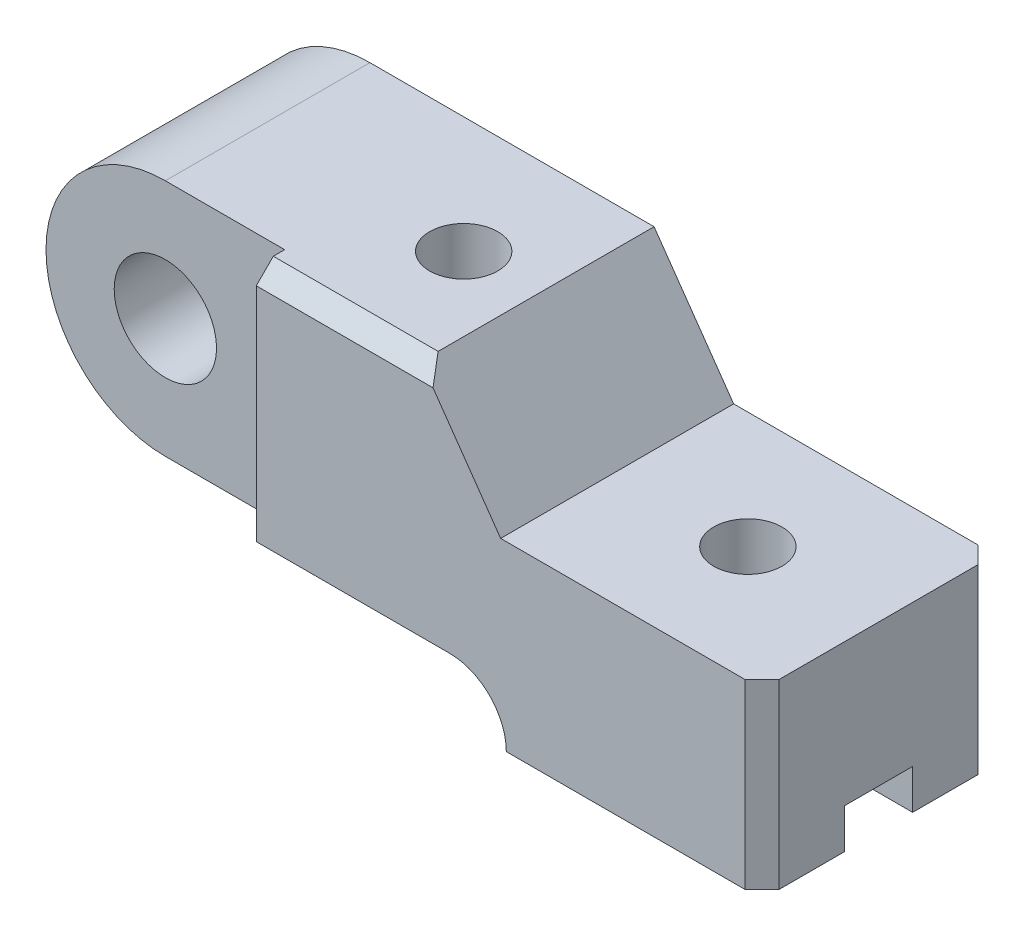
ISO-10303-21;
HEADER;
FILE_DESCRIPTION(('STEP AP214'),'2;1');
FILE_NAME('part.step','',(''),(''),'','','');
FILE_SCHEMA(('AUTOMOTIVE_DESIGN { 1 0 10303 214 1 1 1 1 }'));
ENDSEC;
DATA;
#1=APPLICATION_CONTEXT('core data for automotive mechanical design processes');
#2=APPLICATION_PROTOCOL_DEFINITION('international standard','automotive_design',2000,#1);
#3=PRODUCT_CONTEXT('',#1,'mechanical');
#4=PRODUCT('Part','Part','',(#3));
#5=PRODUCT_RELATED_PRODUCT_CATEGORY('part','',(#4));
#6=PRODUCT_DEFINITION_FORMATION('','',#4);
#7=PRODUCT_DEFINITION_CONTEXT('part definition',#1,'design');
#8=PRODUCT_DEFINITION('design','',#6,#7);
#9=PRODUCT_DEFINITION_SHAPE('','',#8);
#10=(LENGTH_UNIT() NAMED_UNIT(*) SI_UNIT(.MILLI.,.METRE.));
#11=(NAMED_UNIT(*) PLANE_ANGLE_UNIT() SI_UNIT($,.RADIAN.));
#12=(NAMED_UNIT(*) SI_UNIT($,.STERADIAN.) SOLID_ANGLE_UNIT());
#13=UNCERTAINTY_MEASURE_WITH_UNIT(LENGTH_MEASURE(1.E-05),#10,'distance_accuracy_value','');
#14=(GEOMETRIC_REPRESENTATION_CONTEXT(3) GLOBAL_UNCERTAINTY_ASSIGNED_CONTEXT((#13)) GLOBAL_UNIT_ASSIGNED_CONTEXT((#10,
#11,#12)) REPRESENTATION_CONTEXT('',''));
#15=CARTESIAN_POINT('',(0.,0.,0.));
#16=DIRECTION('',(0.,0.,1.));
#17=DIRECTION('',(1.,0.,0.));
#18=AXIS2_PLACEMENT_3D('',#15,#16,#17);
#19=CARTESIAN_POINT('',(0.,0.,20.5));
#20=DIRECTION('',(0.,1.,0.));
#21=DIRECTION('',(-1.,0.,0.));
#22=AXIS2_PLACEMENT_3D('',#19,#20,#21);
#23=PLANE('',#22);
#24=DIRECTION('',(0.,0.,-1.));
#25=VECTOR('',#24,1.);
#26=CARTESIAN_POINT('',(0.,0.,20.5));
#27=LINE('',#26,#25);
#28=CARTESIAN_POINT('',(0.,0.,17.5));
#29=VERTEX_POINT('',#28);
#30=CARTESIAN_POINT('',(0.,0.,6.));
#31=VERTEX_POINT('',#30);
#32=EDGE_CURVE('E195',#29,#31,#27,.T.);
#33=ORIENTED_EDGE('',*,*,#32,.F.);
#34=DIRECTION('',(-0.707106781186546,0.,0.707106781186549));
#35=VECTOR('',#34,1.);
#36=CARTESIAN_POINT('',(-3.,0.,20.5));
#37=LINE('',#36,#35);
#38=CARTESIAN_POINT('',(-3.,0.,20.5));
#39=VERTEX_POINT('',#38);
#40=EDGE_CURVE('E260',#29,#39,#37,.T.);
#41=ORIENTED_EDGE('',*,*,#40,.T.);
#42=DIRECTION('',(1.,0.,0.));
#43=VECTOR('',#42,1.);
#44=CARTESIAN_POINT('',(0.,0.,20.5));
#45=LINE('',#44,#43);
#46=CARTESIAN_POINT('',(-45.,0.,20.5));
#47=VERTEX_POINT('',#46);
#48=EDGE_CURVE('E191',#47,#39,#45,.T.);
#49=ORIENTED_EDGE('',*,*,#48,.F.);
#50=DIRECTION('',(0.,0.,-1.));
#51=VECTOR('',#50,1.);
#52=CARTESIAN_POINT('',(-45.,0.,20.5));
#53=LINE('',#52,#51);
#54=CARTESIAN_POINT('',(-45.,0.,6.));
#55=VERTEX_POINT('',#54);
#56=EDGE_CURVE('E202',#47,#55,#53,.T.);
#57=ORIENTED_EDGE('',*,*,#56,.T.);
#58=DIRECTION('',(1.,0.,0.));
#59=VECTOR('',#58,1.);
#60=CARTESIAN_POINT('',(-131.,0.,6.));
#61=LINE('',#60,#59);
#62=EDGE_CURVE('E326',#55,#31,#61,.T.);
#63=ORIENTED_EDGE('',*,*,#62,.T.);
#64=EDGE_LOOP('',(#33,#41,#49,#57,#63));
#65=FACE_BOUND('',#64,.T.);
#66=ADVANCED_FACE('F41',(#65),#23,.F.);
#67=CARTESIAN_POINT('',(-55.,0.,20.5));
#68=DIRECTION('',(0.,0.,1.));
#69=DIRECTION('',(1.,0.,0.));
#70=AXIS2_PLACEMENT_3D('',#67,#68,#69);
#71=PLANE('',#70);
#72=ORIENTED_EDGE('',*,*,#48,.T.);
#73=DIRECTION('',(0.,1.,0.));
#74=VECTOR('',#73,1.);
#75=CARTESIAN_POINT('',(-3.,32.,20.5));
#76=LINE('',#75,#74);
#77=CARTESIAN_POINT('',(-3.,32.,20.5));
#78=VERTEX_POINT('',#77);
#79=EDGE_CURVE('E255',#39,#78,#76,.T.);
#80=ORIENTED_EDGE('',*,*,#79,.T.);
#81=DIRECTION('',(-1.,0.,0.));
#82=VECTOR('',#81,1.);
#83=CARTESIAN_POINT('',(-45.9968419909216,32.,20.5));
#84=LINE('',#83,#82);
#85=CARTESIAN_POINT('',(-45.9968419909216,32.,20.5));
#86=VERTEX_POINT('',#85);
#87=EDGE_CURVE('E280',#78,#86,#84,.T.);
#88=ORIENTED_EDGE('',*,*,#87,.T.);
#89=DIRECTION('',(-0.573576436351044,0.819152044288993,0.));
#90=VECTOR('',#89,1.);
#91=CARTESIAN_POINT('',(-60.,51.9985821987602,20.5));
#92=LINE('',#91,#90);
#93=CARTESIAN_POINT('',(-57.8993773853709,48.9985821987602,20.5));
#94=VERTEX_POINT('',#93);
#95=EDGE_CURVE('E306',#86,#94,#92,.T.);
#96=ORIENTED_EDGE('',*,*,#95,.T.);
#97=DIRECTION('',(-1.,0.,0.));
#98=VECTOR('',#97,1.);
#99=CARTESIAN_POINT('',(-89.,48.9985821987602,20.5));
#100=LINE('',#99,#98);
#101=CARTESIAN_POINT('',(-89.,48.9985821987602,20.5));
#102=VERTEX_POINT('',#101);
#103=EDGE_CURVE('E253',#94,#102,#100,.T.);
#104=ORIENTED_EDGE('',*,*,#103,.T.);
#105=DIRECTION('',(0.,1.,0.));
#106=VECTOR('',#105,1.);
#107=CARTESIAN_POINT('',(-89.,0.,20.5));
#108=LINE('',#107,#106);
#109=CARTESIAN_POINT('',(-89.,9.99858219876021,20.5));
#110=VERTEX_POINT('',#109);
#111=EDGE_CURVE('E318',#110,#102,#108,.T.);
#112=ORIENTED_EDGE('',*,*,#111,.F.);
#113=DIRECTION('',(1.,0.,0.));
#114=VECTOR('',#113,1.);
#115=CARTESIAN_POINT('',(-110.,9.99858219876022,20.5));
#116=LINE('',#115,#114);
#117=CARTESIAN_POINT('',(-55.1683865037197,9.99858219876023,20.5));
#118=VERTEX_POINT('',#117);
#119=EDGE_CURVE('E313',#110,#118,#116,.T.);
#120=ORIENTED_EDGE('',*,*,#119,.T.);
#121=CARTESIAN_POINT('',(-55.,0.,20.5));
#122=DIRECTION('',(0.,0.,-1.));
#123=DIRECTION('',(1.,0.,0.));
#124=AXIS2_PLACEMENT_3D('',#121,#122,#123);
#125=CIRCLE('',#124,10.);
#126=EDGE_CURVE('E200',#118,#47,#125,.T.);
#127=ORIENTED_EDGE('',*,*,#126,.T.);
#128=EDGE_LOOP('',(#72,#80,#88,#96,#104,#112,#120,#127));
#129=FACE_BOUND('',#128,.T.);
#130=ADVANCED_FACE('F268',(#129),#71,.T.);
#131=CARTESIAN_POINT('',(-55.,0.,-20.5));
#132=DIRECTION('',(0.,0.,1.));
#133=DIRECTION('',(1.,0.,0.));
#134=AXIS2_PLACEMENT_3D('',#131,#132,#133);
#135=PLANE('',#134);
#136=DIRECTION('',(-1.,0.,0.));
#137=VECTOR('',#136,1.);
#138=CARTESIAN_POINT('',(-45.9968419909216,32.,-20.5));
#139=LINE('',#138,#137);
#140=CARTESIAN_POINT('',(-3.00000000000002,32.,-20.5));
#141=VERTEX_POINT('',#140);
#142=CARTESIAN_POINT('',(-45.9968419909216,32.,-20.5));
#143=VERTEX_POINT('',#142);
#144=EDGE_CURVE('E285',#141,#143,#139,.T.);
#145=ORIENTED_EDGE('',*,*,#144,.F.);
#146=DIRECTION('',(0.,-1.,0.));
#147=VECTOR('',#146,1.);
#148=CARTESIAN_POINT('',(-3.00000000000002,0.,-20.5));
#149=LINE('',#148,#147);
#150=CARTESIAN_POINT('',(-3.00000000000002,0.,-20.5));
#151=VERTEX_POINT('',#150);
#152=EDGE_CURVE('E247',#141,#151,#149,.T.);
#153=ORIENTED_EDGE('',*,*,#152,.T.);
#154=DIRECTION('',(1.,0.,0.));
#155=VECTOR('',#154,1.);
#156=CARTESIAN_POINT('',(0.,0.,-20.5));
#157=LINE('',#156,#155);
#158=CARTESIAN_POINT('',(-45.,0.,-20.5));
#159=VERTEX_POINT('',#158);
#160=EDGE_CURVE('E201',#159,#151,#157,.T.);
#161=ORIENTED_EDGE('',*,*,#160,.F.);
#162=CARTESIAN_POINT('',(-55.,0.,-20.5));
#163=DIRECTION('',(0.,0.,-1.));
#164=DIRECTION('',(1.,0.,0.));
#165=AXIS2_PLACEMENT_3D('',#162,#163,#164);
#166=CIRCLE('',#165,10.);
#167=CARTESIAN_POINT('',(-55.1683865037197,9.99858219876023,-20.5));
#168=VERTEX_POINT('',#167);
#169=EDGE_CURVE('E305',#168,#159,#166,.T.);
#170=ORIENTED_EDGE('',*,*,#169,.F.);
#171=DIRECTION('',(1.,0.,0.));
#172=VECTOR('',#171,1.);
#173=CARTESIAN_POINT('',(-55.1683865037197,9.99858219876023,-20.5));
#174=LINE('',#173,#172);
#175=CARTESIAN_POINT('',(-110.,9.99858219876022,-20.5));
#176=VERTEX_POINT('',#175);
#177=EDGE_CURVE('E302',#176,#168,#174,.T.);
#178=ORIENTED_EDGE('',*,*,#177,.F.);
#179=CARTESIAN_POINT('',(-110.,30.9985821987602,-20.5));
#180=DIRECTION('',(0.,0.,1.));
#181=DIRECTION('',(1.,0.,0.));
#182=AXIS2_PLACEMENT_3D('',#179,#180,#181);
#183=CIRCLE('',#182,21.);
#184=CARTESIAN_POINT('',(-110.,51.9985821987602,-20.5));
#185=VERTEX_POINT('',#184);
#186=EDGE_CURVE('E299',#185,#176,#183,.T.);
#187=ORIENTED_EDGE('',*,*,#186,.F.);
#188=DIRECTION('',(-1.,0.,0.));
#189=VECTOR('',#188,1.);
#190=CARTESIAN_POINT('',(-110.,51.9985821987602,-20.5));
#191=LINE('',#190,#189);
#192=CARTESIAN_POINT('',(-60.,51.9985821987602,-20.5));
#193=VERTEX_POINT('',#192);
#194=EDGE_CURVE('E295',#193,#185,#191,.T.);
#195=ORIENTED_EDGE('',*,*,#194,.F.);
#196=DIRECTION('',(-0.573576436351044,0.819152044288993,0.));
#197=VECTOR('',#196,1.);
#198=CARTESIAN_POINT('',(-60.,51.9985821987602,-20.5));
#199=LINE('',#198,#197);
#200=EDGE_CURVE('E286',#143,#193,#199,.T.);
#201=ORIENTED_EDGE('',*,*,#200,.F.);
#202=EDGE_LOOP('',(#145,#153,#161,#170,#178,#187,#195,#201));
#203=FACE_BOUND('',#202,.T.);
#204=CARTESIAN_POINT('',(-110.,30.9985821987602,-20.5));
#205=DIRECTION('',(0.,0.,1.));
#206=DIRECTION('',(1.,0.,0.));
#207=AXIS2_PLACEMENT_3D('',#204,#205,#206);
#208=CIRCLE('',#207,9.);
#209=CARTESIAN_POINT('',(-101.,30.9985821987602,-20.5));
#210=VERTEX_POINT('',#209);
#211=EDGE_CURVE('E234',#210,#210,#208,.T.);
#212=ORIENTED_EDGE('',*,*,#211,.T.);
#213=EDGE_LOOP('',(#212));
#214=FACE_BOUND('',#213,.T.);
#215=ADVANCED_FACE('F284',(#203,#214),#135,.F.);
#216=CARTESIAN_POINT('',(0.,32.,20.5));
#217=DIRECTION('',(-1.,0.,0.));
#218=DIRECTION('',(0.,0.,1.));
#219=AXIS2_PLACEMENT_3D('',#216,#217,#218);
#220=PLANE('',#219);
#221=CARTESIAN_POINT('',(0.,0.,-6.));
#222=VERTEX_POINT('',#221);
#223=CARTESIAN_POINT('',(0.,0.,-17.5));
#224=VERTEX_POINT('',#223);
#225=EDGE_CURVE('E184',#222,#224,#27,.T.);
#226=ORIENTED_EDGE('',*,*,#225,.T.);
#227=DIRECTION('',(0.,1.,0.));
#228=VECTOR('',#227,1.);
#229=CARTESIAN_POINT('',(0.,32.,-17.5));
#230=LINE('',#229,#228);
#231=CARTESIAN_POINT('',(0.,32.,-17.5));
#232=VERTEX_POINT('',#231);
#233=EDGE_CURVE('E245',#224,#232,#230,.T.);
#234=ORIENTED_EDGE('',*,*,#233,.T.);
#235=DIRECTION('',(0.,0.,-1.));
#236=VECTOR('',#235,1.);
#237=CARTESIAN_POINT('',(0.,32.,20.5));
#238=LINE('',#237,#236);
#239=CARTESIAN_POINT('',(0.,32.,17.5));
#240=VERTEX_POINT('',#239);
#241=EDGE_CURVE('E219',#240,#232,#238,.T.);
#242=ORIENTED_EDGE('',*,*,#241,.F.);
#243=DIRECTION('',(0.,-1.,0.));
#244=VECTOR('',#243,1.);
#245=CARTESIAN_POINT('',(0.,0.,17.5));
#246=LINE('',#245,#244);
#247=EDGE_CURVE('E238',#240,#29,#246,.T.);
#248=ORIENTED_EDGE('',*,*,#247,.T.);
#249=ORIENTED_EDGE('',*,*,#32,.T.);
#250=DIRECTION('',(0.,-1.,0.));
#251=VECTOR('',#250,1.);
#252=CARTESIAN_POINT('',(0.,0.,6.));
#253=LINE('',#252,#251);
#254=CARTESIAN_POINT('',(0.,7.,6.));
#255=VERTEX_POINT('',#254);
#256=EDGE_CURVE('E177',#255,#31,#253,.T.);
#257=ORIENTED_EDGE('',*,*,#256,.F.);
#258=DIRECTION('',(0.,0.,1.));
#259=VECTOR('',#258,1.);
#260=CARTESIAN_POINT('',(0.,7.,6.));
#261=LINE('',#260,#259);
#262=CARTESIAN_POINT('',(0.,7.,-6.));
#263=VERTEX_POINT('',#262);
#264=EDGE_CURVE('E186',#263,#255,#261,.T.);
#265=ORIENTED_EDGE('',*,*,#264,.F.);
#266=DIRECTION('',(0.,1.,0.));
#267=VECTOR('',#266,1.);
#268=CARTESIAN_POINT('',(0.,7.,-6.));
#269=LINE('',#268,#267);
#270=EDGE_CURVE('E166',#222,#263,#269,.T.);
#271=ORIENTED_EDGE('',*,*,#270,.F.);
#272=EDGE_LOOP('',(#226,#234,#242,#248,#249,#257,#265,#271));
#273=FACE_BOUND('',#272,.T.);
#274=ADVANCED_FACE('F185',(#273),#220,.F.);
#275=CARTESIAN_POINT('',(-45.9968419909216,32.,20.5));
#276=DIRECTION('',(0.,-1.,0.));
#277=DIRECTION('',(1.,0.,0.));
#278=AXIS2_PLACEMENT_3D('',#275,#276,#277);
#279=PLANE('',#278);
#280=CARTESIAN_POINT('',(-22.9984209954608,32.,0.));
#281=DIRECTION('',(0.,-1.,0.));
#282=DIRECTION('',(1.,0.,0.));
#283=AXIS2_PLACEMENT_3D('',#280,#281,#282);
#284=CIRCLE('',#283,6.);
#285=CARTESIAN_POINT('',(-16.9984209954608,32.,0.));
#286=VERTEX_POINT('',#285);
#287=EDGE_CURVE('E232',#286,#286,#284,.T.);
#288=ORIENTED_EDGE('',*,*,#287,.T.);
#289=EDGE_LOOP('',(#288));
#290=FACE_BOUND('',#289,.T.);
#291=ORIENTED_EDGE('',*,*,#241,.T.);
#292=DIRECTION('',(0.707106781186549,0.,0.707106781186546));
#293=VECTOR('',#292,1.);
#294=CARTESIAN_POINT('',(0.,32.,-17.5));
#295=LINE('',#294,#293);
#296=EDGE_CURVE('E248',#232,#141,#295,.F.);
#297=ORIENTED_EDGE('',*,*,#296,.T.);
#298=ORIENTED_EDGE('',*,*,#144,.T.);
#299=DIRECTION('',(0.,0.,-1.));
#300=VECTOR('',#299,1.);
#301=CARTESIAN_POINT('',(-45.9968419909216,32.,20.5));
#302=LINE('',#301,#300);
#303=EDGE_CURVE('E220',#86,#143,#302,.T.);
#304=ORIENTED_EDGE('',*,*,#303,.F.);
#305=ORIENTED_EDGE('',*,*,#87,.F.);
#306=DIRECTION('',(0.707106781186546,0.,-0.707106781186549));
#307=VECTOR('',#306,1.);
#308=CARTESIAN_POINT('',(-3.,32.,20.5));
#309=LINE('',#308,#307);
#310=EDGE_CURVE('E242',#78,#240,#309,.T.);
#311=ORIENTED_EDGE('',*,*,#310,.T.);
#312=EDGE_LOOP('',(#291,#297,#298,#304,#305,#311));
#313=FACE_BOUND('',#312,.T.);
#314=ADVANCED_FACE('F274',(#290,#313),#279,.F.);
#315=CARTESIAN_POINT('',(-60.,51.9985821987602,20.5));
#316=DIRECTION('',(-0.819152044288993,-0.573576436351044,0.));
#317=DIRECTION('',(0.573576436351044,-0.819152044288993,0.));
#318=AXIS2_PLACEMENT_3D('',#315,#316,#317);
#319=PLANE('',#318);
#320=DIRECTION('',(0.,0.,-1.));
#321=VECTOR('',#320,1.);
#322=CARTESIAN_POINT('',(-60.,51.9985821987602,20.5));
#323=LINE('',#322,#321);
#324=CARTESIAN_POINT('',(-60.,51.9985821987602,17.5));
#325=VERTEX_POINT('',#324);
#326=EDGE_CURVE('E214',#325,#193,#323,.T.);
#327=ORIENTED_EDGE('',*,*,#326,.F.);
#328=DIRECTION('',(0.443712606279655,-0.633687274224641,0.633687274224644));
#329=VECTOR('',#328,1.);
#330=CARTESIAN_POINT('',(-57.3285454230678,48.1833496696123,21.3152325291479));
#331=LINE('',#330,#329);
#332=EDGE_CURVE('E11',#325,#94,#331,.T.);
#333=ORIENTED_EDGE('',*,*,#332,.T.);
#334=ORIENTED_EDGE('',*,*,#95,.F.);
#335=ORIENTED_EDGE('',*,*,#303,.T.);
#336=ORIENTED_EDGE('',*,*,#200,.T.);
#337=EDGE_LOOP('',(#327,#333,#334,#335,#336));
#338=FACE_BOUND('',#337,.T.);
#339=ADVANCED_FACE('F409',(#338),#319,.F.);
#340=CARTESIAN_POINT('',(-110.,51.9985821987602,20.5));
#341=DIRECTION('',(0.,-1.,0.));
#342=DIRECTION('',(0.,0.,-1.));
#343=AXIS2_PLACEMENT_3D('',#340,#341,#342);
#344=PLANE('',#343);
#345=CARTESIAN_POINT('',(-72.9984209954608,51.9985821987602,0.));
#346=DIRECTION('',(0.,1.,0.));
#347=DIRECTION('',(0.,0.,1.));
#348=AXIS2_PLACEMENT_3D('',#345,#346,#347);
#349=CIRCLE('',#348,6.);
#350=CARTESIAN_POINT('',(-72.9984209954608,51.9985821987602,6.));
#351=VERTEX_POINT('',#350);
#352=EDGE_CURVE('E226',#351,#351,#349,.T.);
#353=ORIENTED_EDGE('',*,*,#352,.F.);
#354=EDGE_LOOP('',(#353));
#355=FACE_BOUND('',#354,.T.);
#356=DIRECTION('',(0.,0.,-1.));
#357=VECTOR('',#356,1.);
#358=CARTESIAN_POINT('',(-89.,51.9985821987602,15.5));
#359=LINE('',#358,#357);
#360=CARTESIAN_POINT('',(-89.,51.9985821987602,17.5));
#361=VERTEX_POINT('',#360);
#362=CARTESIAN_POINT('',(-89.,51.9985821987602,15.5));
#363=VERTEX_POINT('',#362);
#364=EDGE_CURVE('E345',#361,#363,#359,.T.);
#365=ORIENTED_EDGE('',*,*,#364,.F.);
#366=DIRECTION('',(1.,0.,0.));
#367=VECTOR('',#366,1.);
#368=CARTESIAN_POINT('',(-60.,51.9985821987602,17.5));
#369=LINE('',#368,#367);
#370=EDGE_CURVE('E49',#361,#325,#369,.T.);
#371=ORIENTED_EDGE('',*,*,#370,.T.);
#372=ORIENTED_EDGE('',*,*,#326,.T.);
#373=ORIENTED_EDGE('',*,*,#194,.T.);
#374=DIRECTION('',(0.,0.,-1.));
#375=VECTOR('',#374,1.);
#376=CARTESIAN_POINT('',(-110.,51.9985821987602,20.5));
#377=LINE('',#376,#375);
#378=CARTESIAN_POINT('',(-110.,51.9985821987602,15.5));
#379=VERTEX_POINT('',#378);
#380=EDGE_CURVE('E213',#379,#185,#377,.T.);
#381=ORIENTED_EDGE('',*,*,#380,.F.);
#382=DIRECTION('',(-1.,0.,0.));
#383=VECTOR('',#382,1.);
#384=CARTESIAN_POINT('',(-131.,51.9985821987602,15.5));
#385=LINE('',#384,#383);
#386=EDGE_CURVE('E347',#363,#379,#385,.T.);
#387=ORIENTED_EDGE('',*,*,#386,.F.);
#388=EDGE_LOOP('',(#365,#371,#372,#373,#381,#387));
#389=FACE_BOUND('',#388,.T.);
#390=ADVANCED_FACE('F410',(#355,#389),#344,.F.);
#391=CARTESIAN_POINT('',(-110.,30.9985821987602,20.5));
#392=DIRECTION('',(0.,0.,-1.));
#393=DIRECTION('',(-1.,0.,0.));
#394=AXIS2_PLACEMENT_3D('',#391,#392,#393);
#395=CYLINDRICAL_SURFACE('',#394,21.);
#396=CARTESIAN_POINT('',(-110.,30.9985821987602,15.5));
#397=DIRECTION('',(0.,0.,-1.));
#398=DIRECTION('',(-1.,0.,0.));
#399=AXIS2_PLACEMENT_3D('',#396,#397,#398);
#400=CIRCLE('',#399,21.);
#401=CARTESIAN_POINT('',(-110.,9.99858219876021,15.5));
#402=VERTEX_POINT('',#401);
#403=EDGE_CURVE('E359',#402,#379,#400,.T.);
#404=ORIENTED_EDGE('',*,*,#403,.T.);
#405=ORIENTED_EDGE('',*,*,#380,.T.);
#406=ORIENTED_EDGE('',*,*,#186,.T.);
#407=DIRECTION('',(0.,0.,-1.));
#408=VECTOR('',#407,1.);
#409=CARTESIAN_POINT('',(-110.,9.99858219876022,20.5));
#410=LINE('',#409,#408);
#411=EDGE_CURVE('E211',#402,#176,#410,.T.);
#412=ORIENTED_EDGE('',*,*,#411,.F.);
#413=EDGE_LOOP('',(#404,#405,#406,#412));
#414=FACE_BOUND('',#413,.T.);
#415=ADVANCED_FACE('F402',(#414),#395,.T.);
#416=CARTESIAN_POINT('',(-55.1683865037197,9.99858219876023,20.5));
#417=DIRECTION('',(0.,1.,0.));
#418=DIRECTION('',(-1.,0.,0.));
#419=AXIS2_PLACEMENT_3D('',#416,#417,#418);
#420=PLANE('',#419);
#421=CARTESIAN_POINT('',(-72.9984209954608,9.99858219876023,0.));
#422=DIRECTION('',(0.,1.,0.));
#423=DIRECTION('',(-1.,0.,0.));
#424=AXIS2_PLACEMENT_3D('',#421,#422,#423);
#425=CIRCLE('',#424,6.);
#426=CARTESIAN_POINT('',(-78.9984209954608,9.99858219876022,0.));
#427=VERTEX_POINT('',#426);
#428=EDGE_CURVE('E227',#427,#427,#425,.T.);
#429=ORIENTED_EDGE('',*,*,#428,.T.);
#430=EDGE_LOOP('',(#429));
#431=FACE_BOUND('',#430,.T.);
#432=DIRECTION('',(0.,0.,-1.));
#433=VECTOR('',#432,1.);
#434=CARTESIAN_POINT('',(-89.,9.99858219876022,20.5));
#435=LINE('',#434,#433);
#436=CARTESIAN_POINT('',(-89.,9.99858219876022,15.5));
#437=VERTEX_POINT('',#436);
#438=EDGE_CURVE('E224',#110,#437,#435,.T.);
#439=ORIENTED_EDGE('',*,*,#438,.T.);
#440=DIRECTION('',(-1.,0.,0.));
#441=VECTOR('',#440,1.);
#442=CARTESIAN_POINT('',(-55.1683865037197,9.99858219876023,15.5));
#443=LINE('',#442,#441);
#444=EDGE_CURVE('E230',#437,#402,#443,.T.);
#445=ORIENTED_EDGE('',*,*,#444,.T.);
#446=ORIENTED_EDGE('',*,*,#411,.T.);
#447=ORIENTED_EDGE('',*,*,#177,.T.);
#448=DIRECTION('',(0.,0.,-1.));
#449=VECTOR('',#448,1.);
#450=CARTESIAN_POINT('',(-55.1683865037197,9.99858219876023,20.5));
#451=LINE('',#450,#449);
#452=EDGE_CURVE('E208',#118,#168,#451,.T.);
#453=ORIENTED_EDGE('',*,*,#452,.F.);
#454=ORIENTED_EDGE('',*,*,#119,.F.);
#455=EDGE_LOOP('',(#439,#445,#446,#447,#453,#454));
#456=FACE_BOUND('',#455,.T.);
#457=ADVANCED_FACE('F319',(#431,#456),#420,.F.);
#458=CARTESIAN_POINT('',(-55.,0.,20.5));
#459=DIRECTION('',(0.,0.,-1.));
#460=DIRECTION('',(-1.,0.,0.));
#461=AXIS2_PLACEMENT_3D('',#458,#459,#460);
#462=CYLINDRICAL_SURFACE('',#461,10.);
#463=DIRECTION('',(0.,0.,-1.));
#464=VECTOR('',#463,1.);
#465=CARTESIAN_POINT('',(-47.8585715714571,7.,20.5));
#466=LINE('',#465,#464);
#467=CARTESIAN_POINT('',(-47.8585715714571,7.,-6.));
#468=VERTEX_POINT('',#467);
#469=CARTESIAN_POINT('',(-47.8585715714571,7.,6.));
#470=VERTEX_POINT('',#469);
#471=EDGE_CURVE('E343',#468,#470,#466,.F.);
#472=ORIENTED_EDGE('',*,*,#471,.T.);
#473=CARTESIAN_POINT('',(-55.,0.,6.));
#474=DIRECTION('',(0.,0.,1.));
#475=DIRECTION('',(1.,0.,0.));
#476=AXIS2_PLACEMENT_3D('',#473,#474,#475);
#477=CIRCLE('',#476,10.);
#478=EDGE_CURVE('E324',#470,#55,#477,.F.);
#479=ORIENTED_EDGE('',*,*,#478,.T.);
#480=ORIENTED_EDGE('',*,*,#56,.F.);
#481=ORIENTED_EDGE('',*,*,#126,.F.);
#482=ORIENTED_EDGE('',*,*,#452,.T.);
#483=ORIENTED_EDGE('',*,*,#169,.T.);
#484=CARTESIAN_POINT('',(-45.,0.,-6.));
#485=VERTEX_POINT('',#484);
#486=EDGE_CURVE('E197',#485,#159,#53,.T.);
#487=ORIENTED_EDGE('',*,*,#486,.F.);
#488=CARTESIAN_POINT('',(-55.,0.,-6.));
#489=DIRECTION('',(0.,0.,-1.));
#490=DIRECTION('',(-1.,0.,0.));
#491=AXIS2_PLACEMENT_3D('',#488,#489,#490);
#492=CIRCLE('',#491,10.);
#493=EDGE_CURVE('E171',#485,#468,#492,.F.);
#494=ORIENTED_EDGE('',*,*,#493,.T.);
#495=EDGE_LOOP('',(#472,#479,#480,#481,#482,#483,#487,#494));
#496=FACE_BOUND('',#495,.T.);
#497=ADVANCED_FACE('F323',(#496),#462,.F.);
#498=ORIENTED_EDGE('',*,*,#160,.T.);
#499=DIRECTION('',(-0.707106781186549,0.,-0.707106781186546));
#500=VECTOR('',#499,1.);
#501=CARTESIAN_POINT('',(0.,0.,-17.5));
#502=LINE('',#501,#500);
#503=EDGE_CURVE('E192',#151,#224,#502,.F.);
#504=ORIENTED_EDGE('',*,*,#503,.T.);
#505=ORIENTED_EDGE('',*,*,#225,.F.);
#506=DIRECTION('',(1.,0.,0.));
#507=VECTOR('',#506,1.);
#508=CARTESIAN_POINT('',(-131.,0.,-6.));
#509=LINE('',#508,#507);
#510=EDGE_CURVE('E164',#485,#222,#509,.T.);
#511=ORIENTED_EDGE('',*,*,#510,.F.);
#512=ORIENTED_EDGE('',*,*,#486,.T.);
#513=EDGE_LOOP('',(#498,#504,#505,#511,#512));
#514=FACE_BOUND('',#513,.T.);
#515=ADVANCED_FACE('F193',(#514),#23,.F.);
#516=CARTESIAN_POINT('',(-110.,30.9985821987602,20.5));
#517=DIRECTION('',(0.,0.,-1.));
#518=DIRECTION('',(-1.,0.,0.));
#519=AXIS2_PLACEMENT_3D('',#516,#517,#518);
#520=CYLINDRICAL_SURFACE('',#519,9.);
#521=CARTESIAN_POINT('',(-110.,30.9985821987602,15.5));
#522=DIRECTION('',(0.,0.,-1.));
#523=DIRECTION('',(-1.,0.,0.));
#524=AXIS2_PLACEMENT_3D('',#521,#522,#523);
#525=CIRCLE('',#524,9.);
#526=CARTESIAN_POINT('',(-119.,30.9985821987602,15.5));
#527=VERTEX_POINT('',#526);
#528=EDGE_CURVE('E221',#527,#527,#525,.T.);
#529=ORIENTED_EDGE('',*,*,#528,.F.);
#530=EDGE_LOOP('',(#529));
#531=FACE_BOUND('',#530,.T.);
#532=ORIENTED_EDGE('',*,*,#211,.F.);
#533=EDGE_LOOP('',(#532));
#534=FACE_BOUND('',#533,.T.);
#535=ADVANCED_FACE('F388',(#531,#534),#520,.F.);
#536=CARTESIAN_POINT('',(-89.,0.,15.5));
#537=DIRECTION('',(1.,0.,0.));
#538=DIRECTION('',(0.,0.,-1.));
#539=AXIS2_PLACEMENT_3D('',#536,#537,#538);
#540=PLANE('',#539);
#541=ORIENTED_EDGE('',*,*,#111,.T.);
#542=DIRECTION('',(0.,0.707106781186546,-0.707106781186549));
#543=VECTOR('',#542,1.);
#544=CARTESIAN_POINT('',(-89.,48.9985821987602,20.5));
#545=LINE('',#544,#543);
#546=EDGE_CURVE('E62',#102,#361,#545,.T.);
#547=ORIENTED_EDGE('',*,*,#546,.T.);
#548=ORIENTED_EDGE('',*,*,#364,.T.);
#549=DIRECTION('',(0.,1.,0.));
#550=VECTOR('',#549,1.);
#551=CARTESIAN_POINT('',(-89.,0.,15.5));
#552=LINE('',#551,#550);
#553=EDGE_CURVE('E349',#437,#363,#552,.T.);
#554=ORIENTED_EDGE('',*,*,#553,.F.);
#555=ORIENTED_EDGE('',*,*,#438,.F.);
#556=EDGE_LOOP('',(#541,#547,#548,#554,#555));
#557=FACE_BOUND('',#556,.T.);
#558=ADVANCED_FACE('F376',(#557),#540,.F.);
#559=CARTESIAN_POINT('',(-131.,0.,15.5));
#560=DIRECTION('',(0.,0.,-1.));
#561=DIRECTION('',(-1.,0.,0.));
#562=AXIS2_PLACEMENT_3D('',#559,#560,#561);
#563=PLANE('',#562);
#564=ORIENTED_EDGE('',*,*,#528,.T.);
#565=EDGE_LOOP('',(#564));
#566=FACE_BOUND('',#565,.T.);
#567=ORIENTED_EDGE('',*,*,#403,.F.);
#568=ORIENTED_EDGE('',*,*,#444,.F.);
#569=ORIENTED_EDGE('',*,*,#553,.T.);
#570=ORIENTED_EDGE('',*,*,#386,.T.);
#571=EDGE_LOOP('',(#567,#568,#569,#570));
#572=FACE_BOUND('',#571,.T.);
#573=ADVANCED_FACE('F364',(#566,#572),#563,.F.);
#574=CARTESIAN_POINT('',(-22.9984209954608,0.,0.));
#575=DIRECTION('',(0.,1.,0.));
#576=DIRECTION('',(0.,0.,1.));
#577=AXIS2_PLACEMENT_3D('',#574,#575,#576);
#578=CYLINDRICAL_SURFACE('',#577,6.);
#579=CARTESIAN_POINT('',(-22.9984209954608,7.,0.));
#580=DIRECTION('',(0.,1.,0.));
#581=DIRECTION('',(0.,0.,1.));
#582=AXIS2_PLACEMENT_3D('',#579,#580,#581);
#583=CIRCLE('',#582,6.);
#584=CARTESIAN_POINT('',(-22.9984209954608,7.,-6.));
#585=VERTEX_POINT('',#584);
#586=CARTESIAN_POINT('',(-22.9984209954608,7.,6.));
#587=VERTEX_POINT('',#586);
#588=EDGE_CURVE('E237',#585,#587,#583,.F.);
#589=ORIENTED_EDGE('',*,*,#588,.T.);
#590=EDGE_CURVE('E239',#587,#585,#583,.F.);
#591=ORIENTED_EDGE('',*,*,#590,.T.);
#592=EDGE_LOOP('',(#589,#591));
#593=FACE_BOUND('',#592,.T.);
#594=ORIENTED_EDGE('',*,*,#287,.F.);
#595=EDGE_LOOP('',(#594));
#596=FACE_BOUND('',#595,.T.);
#597=ADVANCED_FACE('F362',(#593,#596),#578,.F.);
#598=CARTESIAN_POINT('',(-72.9984209954608,0.,0.));
#599=DIRECTION('',(0.,1.,0.));
#600=DIRECTION('',(0.,0.,1.));
#601=AXIS2_PLACEMENT_3D('',#598,#599,#600);
#602=CYLINDRICAL_SURFACE('',#601,6.);
#603=ORIENTED_EDGE('',*,*,#352,.T.);
#604=EDGE_LOOP('',(#603));
#605=FACE_BOUND('',#604,.T.);
#606=ORIENTED_EDGE('',*,*,#428,.F.);
#607=EDGE_LOOP('',(#606));
#608=FACE_BOUND('',#607,.T.);
#609=ADVANCED_FACE('F365',(#605,#608),#602,.F.);
#610=CARTESIAN_POINT('',(-131.,0.,6.));
#611=DIRECTION('',(0.,0.,1.));
#612=DIRECTION('',(1.,0.,0.));
#613=AXIS2_PLACEMENT_3D('',#610,#611,#612);
#614=PLANE('',#613);
#615=DIRECTION('',(1.,0.,0.));
#616=VECTOR('',#615,1.);
#617=CARTESIAN_POINT('',(-131.,7.,6.));
#618=LINE('',#617,#616);
#619=EDGE_CURVE('E328',#470,#587,#618,.T.);
#620=ORIENTED_EDGE('',*,*,#619,.T.);
#621=EDGE_CURVE('E334',#587,#255,#618,.T.);
#622=ORIENTED_EDGE('',*,*,#621,.T.);
#623=ORIENTED_EDGE('',*,*,#256,.T.);
#624=ORIENTED_EDGE('',*,*,#62,.F.);
#625=ORIENTED_EDGE('',*,*,#478,.F.);
#626=EDGE_LOOP('',(#620,#622,#623,#624,#625));
#627=FACE_BOUND('',#626,.T.);
#628=ADVANCED_FACE('F332',(#627),#614,.F.);
#629=CARTESIAN_POINT('',(-131.,7.,6.));
#630=DIRECTION('',(0.,1.,0.));
#631=DIRECTION('',(0.,0.,1.));
#632=AXIS2_PLACEMENT_3D('',#629,#630,#631);
#633=PLANE('',#632);
#634=DIRECTION('',(1.,0.,0.));
#635=VECTOR('',#634,1.);
#636=CARTESIAN_POINT('',(-131.,7.,-6.));
#637=LINE('',#636,#635);
#638=EDGE_CURVE('E336',#468,#585,#637,.T.);
#639=ORIENTED_EDGE('',*,*,#638,.T.);
#640=ORIENTED_EDGE('',*,*,#590,.F.);
#641=ORIENTED_EDGE('',*,*,#619,.F.);
#642=ORIENTED_EDGE('',*,*,#471,.F.);
#643=EDGE_LOOP('',(#639,#640,#641,#642));
#644=FACE_BOUND('',#643,.T.);
#645=ADVANCED_FACE('F534',(#644),#633,.F.);
#646=EDGE_CURVE('E179',#585,#263,#637,.T.);
#647=ORIENTED_EDGE('',*,*,#646,.T.);
#648=ORIENTED_EDGE('',*,*,#264,.T.);
#649=ORIENTED_EDGE('',*,*,#621,.F.);
#650=ORIENTED_EDGE('',*,*,#588,.F.);
#651=EDGE_LOOP('',(#647,#648,#649,#650));
#652=FACE_BOUND('',#651,.T.);
#653=ADVANCED_FACE('F543',(#652),#633,.F.);
#654=CARTESIAN_POINT('',(-131.,7.,-6.));
#655=DIRECTION('',(0.,0.,-1.));
#656=DIRECTION('',(-1.,0.,0.));
#657=AXIS2_PLACEMENT_3D('',#654,#655,#656);
#658=PLANE('',#657);
#659=ORIENTED_EDGE('',*,*,#510,.T.);
#660=ORIENTED_EDGE('',*,*,#270,.T.);
#661=ORIENTED_EDGE('',*,*,#646,.F.);
#662=ORIENTED_EDGE('',*,*,#638,.F.);
#663=ORIENTED_EDGE('',*,*,#493,.F.);
#664=EDGE_LOOP('',(#659,#660,#661,#662,#663));
#665=FACE_BOUND('',#664,.T.);
#666=ADVANCED_FACE('F170',(#665),#658,.F.);
#667=CARTESIAN_POINT('',(0.,32.,-17.5));
#668=DIRECTION('',(-0.707106781186546,0.,0.707106781186549));
#669=DIRECTION('',(0.,1.,0.));
#670=AXIS2_PLACEMENT_3D('',#667,#668,#669);
#671=PLANE('',#670);
#672=ORIENTED_EDGE('',*,*,#503,.F.);
#673=ORIENTED_EDGE('',*,*,#152,.F.);
#674=ORIENTED_EDGE('',*,*,#296,.F.);
#675=ORIENTED_EDGE('',*,*,#233,.F.);
#676=EDGE_LOOP('',(#672,#673,#674,#675));
#677=FACE_BOUND('',#676,.T.);
#678=ADVANCED_FACE('F276',(#677),#671,.F.);
#679=CARTESIAN_POINT('',(-3.,0.,20.5));
#680=DIRECTION('',(0.707106781186549,0.,0.707106781186546));
#681=DIRECTION('',(0.,-1.,0.));
#682=AXIS2_PLACEMENT_3D('',#679,#680,#681);
#683=PLANE('',#682);
#684=ORIENTED_EDGE('',*,*,#40,.F.);
#685=ORIENTED_EDGE('',*,*,#247,.F.);
#686=ORIENTED_EDGE('',*,*,#310,.F.);
#687=ORIENTED_EDGE('',*,*,#79,.F.);
#688=EDGE_LOOP('',(#684,#685,#686,#687));
#689=FACE_BOUND('',#688,.T.);
#690=ADVANCED_FACE('F275',(#689),#683,.T.);
#691=CARTESIAN_POINT('',(-55.,48.9985821987602,20.5));
#692=DIRECTION('',(0.,0.707106781186549,0.707106781186546));
#693=DIRECTION('',(1.,0.,0.));
#694=AXIS2_PLACEMENT_3D('',#691,#692,#693);
#695=PLANE('',#694);
#696=ORIENTED_EDGE('',*,*,#332,.F.);
#697=ORIENTED_EDGE('',*,*,#370,.F.);
#698=ORIENTED_EDGE('',*,*,#546,.F.);
#699=ORIENTED_EDGE('',*,*,#103,.F.);
#700=EDGE_LOOP('',(#696,#697,#698,#699));
#701=FACE_BOUND('',#700,.T.);
#702=ADVANCED_FACE('F42',(#701),#695,.T.);
#703=CLOSED_SHELL('',(#66,#130,#215,#274,#314,#339,#390,#415,#457,#497,#515,#535,#558,#573,#597,
#609,#628,#645,#653,#666,#678,#690,#702));
#704=MANIFOLD_SOLID_BREP('B2',#703);
#705=ADVANCED_BREP_SHAPE_REPRESENTATION('',(#18,#704),#14);
#706=SHAPE_DEFINITION_REPRESENTATION(#9,#705);
ENDSEC;
END-ISO-10303-21;
